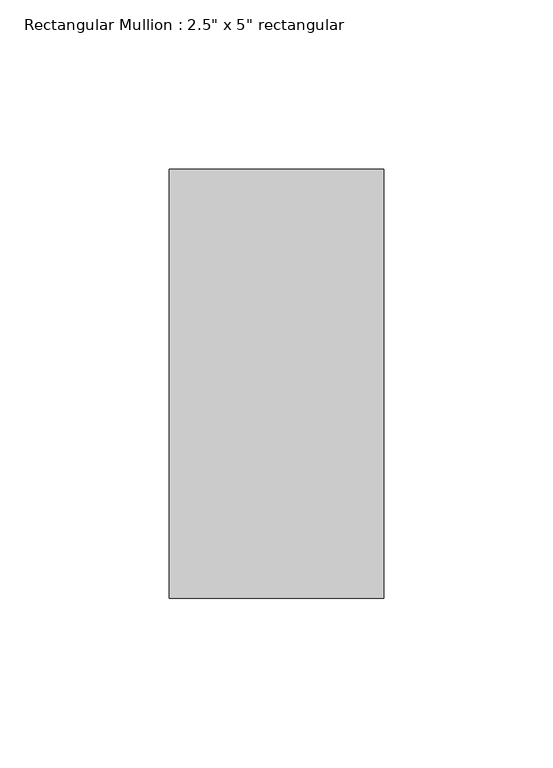
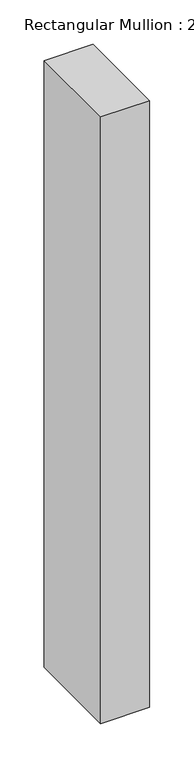
"""IFC4 building model written with IfcOpenShell, lengths in millimetres: member geometry."""

from ifc_helpers import new_model, si_unit, frame, origin, place, context, project, spatial, polyline, outline, extrude, source, transform, mapped, element, save


def member_655cfd9b(model_context):
    return source(origin(), model_context, "Body", "SweptSolid", [
        extrude(outline(polyline([(31.75, 63.5), (31.75, -63.5), (-31.75, -63.5), (-31.75, 63.5), (31.75, 63.5)])), frame((0.0, 0.0, -832.4388769), z_axis=(0.0, 0.0, 1.0), x_axis=(1.0, 0.0, 0.0)), (0.0, 0.0, 1.0), 832.4388769),
    ])


if __name__ == "__main__":
    model = new_model("IFC4")
    model_context = context("Model", 3, world=origin())
    ifc_project = project(units=[si_unit("LENGTHUNIT", "METRE", prefix="MILLI")], contexts=[model_context])
    site = spatial("IfcSite", under=ifc_project)
    building = spatial("IfcBuilding", under=site)
    placement = place(None, origin())
    member_shape = member_655cfd9b(model_context)
    element("IfcMember", 1, ObjectType="Rectangular Mullion : 2.5\" x 5\" rectangular", at=placement, inside=building, context=model_context, shape_type="MappedRepresentation", body=[
        mapped(member_shape, transform((0.0, 0.0, 0.0), x_axis=(1.0, 0.0, 0.0), y_axis=(0.0, 1.0, 0.0), z_axis=(0.0, 0.0, 1.0))),
    ])
    save(model, "model.ifc")

# Revit data of these elements
# Type "Rectangular Mullion : 2.5\" x 5\" rectangular"
#   built-in parameter 1007304 = 0.416667 (stored number, unit not read)
#   built-in parameter 1007301 = 0.104167 (stored number, unit not read)
#   built-in parameter 1007300 = 0.104167 (stored number, unit not read)
# Element 1 (IfcMember, "Rectangular Mullion : 2.5\" x 5\" rectangular")
#   Materials on its faces: "Aluminum"
# Materials
#   "Aluminum": class "Metal", colour RGB 247 247 247, transparency 0, Description = "Aluminum 6061", Cost = 0
